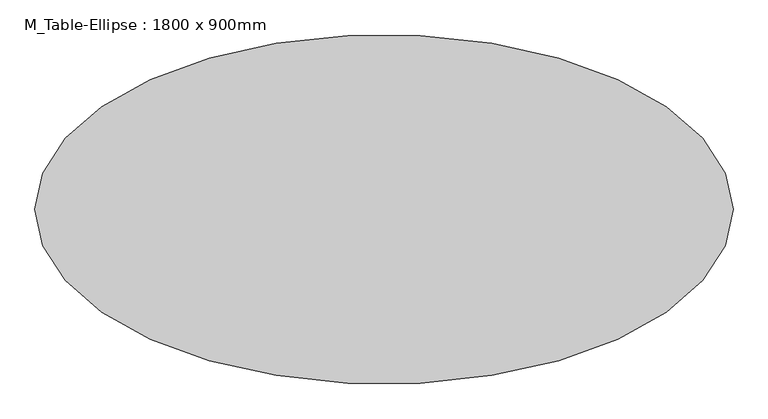
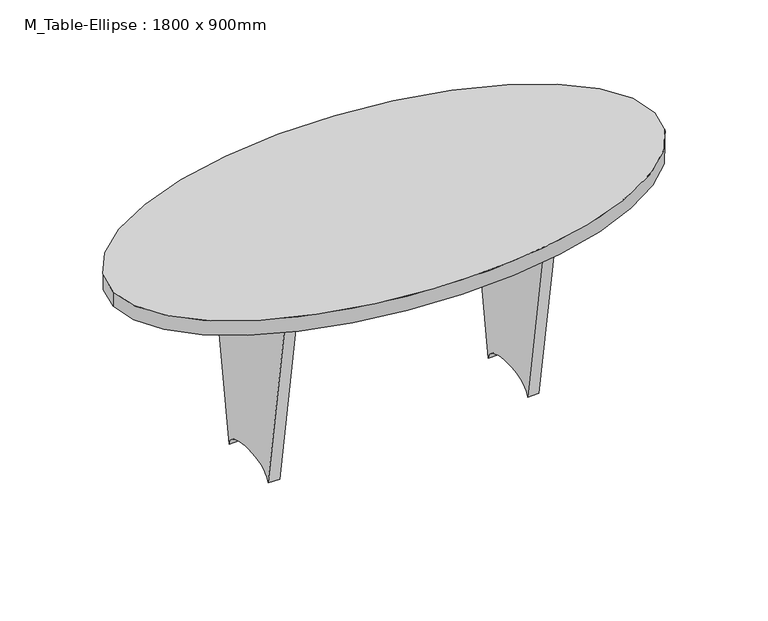
"""IFC4 building model written with IfcOpenShell, lengths in millimetres: furniture geometry, M_Table-Ellipse : 1800 x 900mm."""

from ifc_helpers import new_model, si_unit, point, frame, origin, place, context, project, spatial, ellipse_curve, trimmed, source, transform, mapped, element, save
from ifc_brep_helpers import plane_surface, extruded_surface, advanced_brep


def m_table_ellipse_1800_x_900mm_fd46d5a5(model_context):
    return source(origin(), model_context, "Body", "AdvancedBrep", [
        advanced_brep(
        [(-411.9, 19.05, 709.2), (411.9, 19.05, 709.2), (411.9, 19.05, 472.8), (-411.9, 19.05, 472.8), (-411.9, -19.05, 709.2), (-411.9, -19.05, 472.8), (411.9, -19.05, 472.8), (411.9, -19.05, 709.2)],
        [
            (0, 1),
            (1, 2),
            (2, 3, ellipse_curve(frame((0.0, 19.05, 472.8), z_axis=(0.0, -1.0, 0.0), x_axis=(1.0, 0.0, 0.0)), 411.9, 101.6)),
            (3, 0),
            (4, 5),
            (5, 6, ellipse_curve(frame((0.0, -19.05, 472.8), z_axis=(0.0, 1.0, 0.0), x_axis=(1.0, 0.0, 0.0)), 411.9, 101.6)),
            (6, 7),
            (7, 4),
            (0, 4),
            (7, 1),
            (6, 2),
            (5, 3),
        ],
        [
            plane_surface(frame((-411.9, 19.05, 709.2), z_axis=(0.0, 1.0, 0.0), x_axis=(1.0, 0.0, 0.0))),
            plane_surface(frame((-411.9, -19.05, 709.2), z_axis=(0.0, -1.0, 0.0), x_axis=(-1.0, 0.0, 0.0))),
            plane_surface(frame((-411.9, 19.05, 709.2), z_axis=(0.0, 0.0, 1.0), x_axis=(0.0, -1.0, 0.0))),
            plane_surface(frame((411.9, 19.05, 709.2), z_axis=(1.0, 0.0, 0.0), x_axis=(0.0, -1.0, 0.0))),
            extruded_surface(trimmed(ellipse_curve(frame((0.0, -57.15, 472.8), z_axis=(0.0, -1.0, 0.0), x_axis=(1.0, 0.0, 0.0)), 411.9, 101.6), [point((411.9, -57.15, 472.8))], [point((-411.9, -57.15, 472.8))], True, "CARTESIAN"), (0.0, 38.099999999999994, 0.0), 38.099999999999994),
            plane_surface(frame((-411.9, 19.05, 472.8), z_axis=(-1.0, 0.0, 0.0), x_axis=(0.0, -1.0, 0.0))),
        ],
        [
            (0, [[1, 2, 3, 4]]),
            (1, [[5, 6, 7, 8]]),
            (2, [[-1, 9, -8, 10]]),
            (3, [[-2, -10, -7, 11]]),
            (4, [[-3, -11, -6, 12]]),
            (5, [[-4, -12, -5, -9]]),
        ],
    ),
        advanced_brep(
        [(450.0, 225.0, 709.2), (450.0, -225.0, 709.2), (450.0, -112.5, 0.0), (450.0, 112.5, 0.0), (411.9, 225.0, 709.2), (411.9, 112.5, 0.0), (411.9, -112.5, 0.0), (411.9, -225.0, 709.2)],
        [
            (0, 1),
            (1, 2),
            (2, 3, ellipse_curve(frame((450.0, 0.0, 0.0), z_axis=(-1.0, 0.0, 0.0), x_axis=(0.0, 1.0, 0.0)), 112.5, 50.8)),
            (3, 0),
            (4, 5),
            (5, 6, ellipse_curve(frame((411.9, 0.0, 0.0), z_axis=(1.0, 0.0, 0.0), x_axis=(0.0, 1.0, 0.0)), 112.5, 50.8)),
            (6, 7),
            (7, 4),
            (0, 4),
            (7, 1),
            (6, 2),
            (5, 3),
        ],
        [
            plane_surface(frame((450.0, -225.0, 709.2), z_axis=(1.0, 0.0, 0.0), x_axis=(0.0, -1.0, 0.0))),
            plane_surface(frame((411.9, -225.0, 709.2), z_axis=(-1.0, 0.0, 0.0), x_axis=(0.0, 1.0, 0.0))),
            plane_surface(frame((450.0, 225.0, 709.2), z_axis=(0.0, 0.0, 1.0), x_axis=(-1.0, 0.0, 0.0))),
            plane_surface(frame((450.0, -225.0, 709.2), z_axis=(0.0, -0.9876509250759588, -0.1566705147645943), x_axis=(-1.0, 0.0, 0.0))),
            extruded_surface(trimmed(ellipse_curve(frame((373.8, 0.0, 0.0), z_axis=(-1.0, 0.0, 0.0), x_axis=(0.0, 1.0, 0.0)), 112.5, 50.8), [point((373.8, -112.5, 0.0))], [point((373.8, 112.5, 0.0))], True, "CARTESIAN"), (38.099999999999966, 0.0, 0.0), 38.099999999999966),
            plane_surface(frame((450.0, 112.5, 0.0), z_axis=(0.0, 0.9876509250759595, -0.1566705147645892), x_axis=(-1.0, 0.0, 0.0))),
        ],
        [
            (0, [[1, 2, 3, 4]]),
            (1, [[5, 6, 7, 8]]),
            (2, [[-1, 9, -8, 10]]),
            (3, [[-2, -10, -7, 11]]),
            (4, [[-3, -11, -6, 12]]),
            (5, [[-4, -12, -5, -9]]),
        ],
    ),
        advanced_brep(
        [(-411.9, 225.0, 709.2), (-411.9, -225.0, 709.2), (-411.9, -112.5, 0.0), (-411.9, 112.5, 0.0), (-450.0, 225.0, 709.2), (-450.0, 112.5, 0.0), (-450.0, -112.5, 0.0), (-450.0, -225.0, 709.2)],
        [
            (0, 1),
            (1, 2),
            (2, 3, ellipse_curve(frame((-411.9, 0.0, 0.0), z_axis=(-1.0, 0.0, 0.0), x_axis=(0.0, 1.0, 0.0)), 112.5, 50.8)),
            (3, 0),
            (4, 5),
            (5, 6, ellipse_curve(frame((-450.0, 0.0, 0.0), z_axis=(1.0, 0.0, 0.0), x_axis=(0.0, 1.0, 0.0)), 112.5, 50.8)),
            (6, 7),
            (7, 4),
            (0, 4),
            (7, 1),
            (6, 2),
            (5, 3),
        ],
        [
            plane_surface(frame((-411.9, -225.0, 709.2), z_axis=(1.0, 0.0, 0.0), x_axis=(0.0, -1.0, 0.0))),
            plane_surface(frame((-450.0, -225.0, 709.2), z_axis=(-1.0, 0.0, 0.0), x_axis=(0.0, 1.0, 0.0))),
            plane_surface(frame((-411.9, 225.0, 709.2), z_axis=(0.0, 0.0, 1.0), x_axis=(-1.0, 0.0, 0.0))),
            plane_surface(frame((-411.9, -225.0, 709.2), z_axis=(0.0, -0.9876509250759585, -0.15667051476459606), x_axis=(-1.0, 0.0, 0.0))),
            extruded_surface(trimmed(ellipse_curve(frame((-488.1, 0.0, 0.0), z_axis=(-1.0, 0.0, 0.0), x_axis=(0.0, 1.0, 0.0)), 112.5, 50.8), [point((-488.1, -112.5, 0.0))], [point((-488.1, 112.5, 0.0))], True, "CARTESIAN"), (38.10000000000002, 0.0, 0.0), 38.10000000000002),
            plane_surface(frame((-411.9, 112.5, 0.0), z_axis=(0.0, 0.9876509250759599, -0.1566705147645873), x_axis=(-1.0, 0.0, 0.0))),
        ],
        [
            (0, [[1, 2, 3, 4]]),
            (1, [[5, 6, 7, 8]]),
            (2, [[-1, 9, -8, 10]]),
            (3, [[-2, -10, -7, 11]]),
            (4, [[-3, -11, -6, 12]]),
            (5, [[-4, -12, -5, -9]]),
        ],
    ),
        advanced_brep(
        [(-900.0, 0.0, 760.0), (900.0, 0.0, 760.0), (-900.0, 0.0, 709.2), (900.0, 0.0, 709.2)],
        [
            (0, 1, ellipse_curve(frame((0.0, 0.0, 760.0), z_axis=(0.0, 0.0, 1.0), x_axis=(1.0, 0.0, 0.0)), 900.0, 450.0)),
            (1, 0, ellipse_curve(frame((0.0, 0.0, 760.0), z_axis=(0.0, 0.0, 1.0), x_axis=(1.0, 0.0, 0.0)), 900.0, 450.0)),
            (2, 3, ellipse_curve(frame((0.0, 0.0, 709.2), z_axis=(0.0, 0.0, -1.0), x_axis=(1.0, 0.0, 0.0)), 900.0, 450.0)),
            (3, 2, ellipse_curve(frame((0.0, 0.0, 709.2), z_axis=(0.0, 0.0, -1.0), x_axis=(1.0, 0.0, 0.0)), 900.0, 450.0)),
            (0, 2),
            (3, 1),
        ],
        [
            plane_surface(frame((900.0, 0.0, 760.0), z_axis=(0.0, 0.0, 1.0), x_axis=(0.0, 1.0, 0.0))),
            plane_surface(frame((900.0, 0.0, 709.2), z_axis=(0.0, 0.0, -1.0), x_axis=(0.0, -1.0, 0.0))),
            extruded_surface(trimmed(ellipse_curve(frame((0.0, 0.0, 658.4), z_axis=(0.0, 0.0, 1.0), x_axis=(1.0, 0.0, 0.0)), 900.0, 450.0), [point((-900.0, 0.0, 658.4))], [point((900.0, 0.0, 658.4))], True, "CARTESIAN"), (0.0, 0.0, 50.80000000000007), 50.80000000000007),
            extruded_surface(trimmed(ellipse_curve(frame((0.0, 0.0, 658.4), z_axis=(0.0, 0.0, 1.0), x_axis=(1.0, 0.0, 0.0)), 900.0, 450.0), [point((900.0, 0.0, 658.4))], [point((-900.0, 0.0, 658.4))], True, "CARTESIAN"), (0.0, 0.0, 50.80000000000007), 50.80000000000007),
        ],
        [
            (0, [[1, 2]]),
            (1, [[3, 4]]),
            (2, [[-1, 5, -4, 6]]),
            (3, [[-2, -6, -3, -5]]),
        ],
    ),
    ])


if __name__ == "__main__":
    model = new_model("IFC4")
    model_context = context("Model", 3, world=origin())
    ifc_project = project(units=[si_unit("LENGTHUNIT", "METRE", prefix="MILLI")], contexts=[model_context])
    site = spatial("IfcSite", under=ifc_project)
    building = spatial("IfcBuilding", under=site)
    placement = place(None, origin())
    m_table_ellipse_1800_x_900mm_shape = m_table_ellipse_1800_x_900mm_fd46d5a5(model_context)
    element("IfcFurniture", 1, ObjectType="M_Table-Ellipse : 1800 x 900mm", at=placement, inside=building, context=model_context, shape_type="MappedRepresentation", body=[
        mapped(m_table_ellipse_1800_x_900mm_shape, transform((0.0, 0.0, 0.0), x_axis=(1.0, 0.0, 0.0), y_axis=(0.0, 1.0, 0.0), z_axis=(0.0, 0.0, 1.0))),
    ])
    save(model, "model.ifc")

# Revit data of these elements
# Type "M_Table-Ellipse : 1800 x 900mm"
#   Half Width = 450 mm
#   Half Length = 900 mm
#   Height = 760 mm
#   Length = 1800 mm
#   Width = 900 mm
#   Base Material = Birch
#   Top Material = Laminate - Black
#   Default Elevation = 0
#   Assembly Code = ""
# Element 1 (IfcFurniture, "M_Table-Ellipse : 1800 x 900mm")
#   Materials on its faces: "Birch", "Laminate - Black"
# Materials
#   "Birch": class "Wood", colour RGB 224 178 126, transparency 0, Description = "Betula Alleghaniensis", Cost = 0
#   "Laminate - Black": colour RGB 0 0 0, transparency 0
